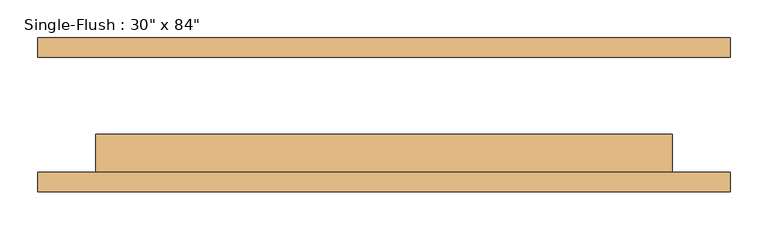
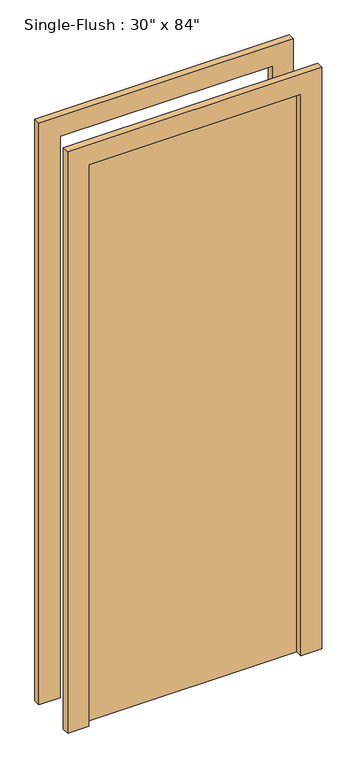
"""IFC4 building model written with IfcOpenShell, lengths in millimetres: door geometry."""

from ifc_helpers import new_model, si_unit, frame, origin, origin_with_axes, place, context, project, spatial, polyline, outline, extrude, source, transform, mapped, element, save


def door_e2b13fe9(model_context):
    return source(origin(), model_context, "Body", "SweptSolid", [
        extrude(outline(polyline([(2209.8, -457.2), (0.0, -457.2), (0.0, -381.0), (2133.6, -381.0), (2133.6, 381.0), (0.0, 381.0), (0.0, 457.2), (2209.8, 457.2), (2209.8, -457.2)])), frame((0.0, -101.6, 0.0), z_axis=(0.0, 1.0, 0.0), x_axis=(0.0, 0.0, 1.0)), (0.0, 0.0, 1.0), 25.4),
        extrude(outline(polyline([(2209.8, 457.2), (2209.8, -457.2), (0.0, -457.2), (0.0, -381.0), (2133.6, -381.0), (2133.6, 381.0), (0.0, 381.0), (0.0, 457.2), (2209.8, 457.2)])), frame((0.0, 76.2, 0.0), z_axis=(0.0, 1.0, 0.0), x_axis=(0.0, 0.0, 1.0)), (0.0, 0.0, 1.0), 25.4),
        extrude(outline(polyline([(381.0, -25.4), (381.0, -76.2), (-381.0, -76.2), (-381.0, -25.4), (381.0, -25.4)])), origin_with_axes(), (0.0, 0.0, 1.0), 2133.6),
    ])


if __name__ == "__main__":
    model = new_model("IFC4")
    model_context = context("Model", 3, world=origin())
    ifc_project = project(units=[si_unit("LENGTHUNIT", "METRE", prefix="MILLI")], contexts=[model_context])
    site = spatial("IfcSite", under=ifc_project)
    building = spatial("IfcBuilding", under=site)
    placement = place(None, origin())
    door_shape = door_e2b13fe9(model_context)
    element("IfcDoor", 1, ObjectType="Single-Flush : 30\" x 84\"", at=placement, inside=building, context=model_context, shape_type="MappedRepresentation", body=[
        mapped(door_shape, transform((0.0, 0.0, 0.0), x_axis=(1.0, 0.0, 0.0), y_axis=(0.0, 1.0, 0.0), z_axis=(0.0, 0.0, 1.0))),
    ])
    save(model, "model.ifc")

# Revit data of these elements
# Type "Single-Flush : 30\" x 84\""
#   Type Mark = "1"
#   Construction Type Id = "MDOOR"
#   Assembly Code = "C1020"
#   Analytic Construction = "Metal"
#   Thickness = 0' - 2"
#   Heat Transfer Coefficient (U) = 0.651978 BTU/(h·ft²·°F)
#   Height = 7' - 0"
#   Trim Projection Ext = 0' - 1"
#   Trim Projection Int = 0' - 1"
#   Trim Width = 0' - 3"
#   Width = 2' - 6"
#   Define Thermal Properties by = 1
#   Door Material = Door - Panel
#   Frame Material = Door - Frame
#   Visual Light Transmittance = 0
#   Solar Heat Gain Coefficient = 0
#   Function = (empty or 0)
#   Wall Closure = (empty or 0)
# Element 1 (IfcDoor, "Single-Flush : 30\" x 84\"")
#   Materials on its faces: "Door - Frame", "Door - Panel"
# Materials
#   "Door - Panel": class "Wood", colour RGB 210 159 95, transparency 0
#   "Door - Frame": colour RGB 118 70 51, transparency 0
